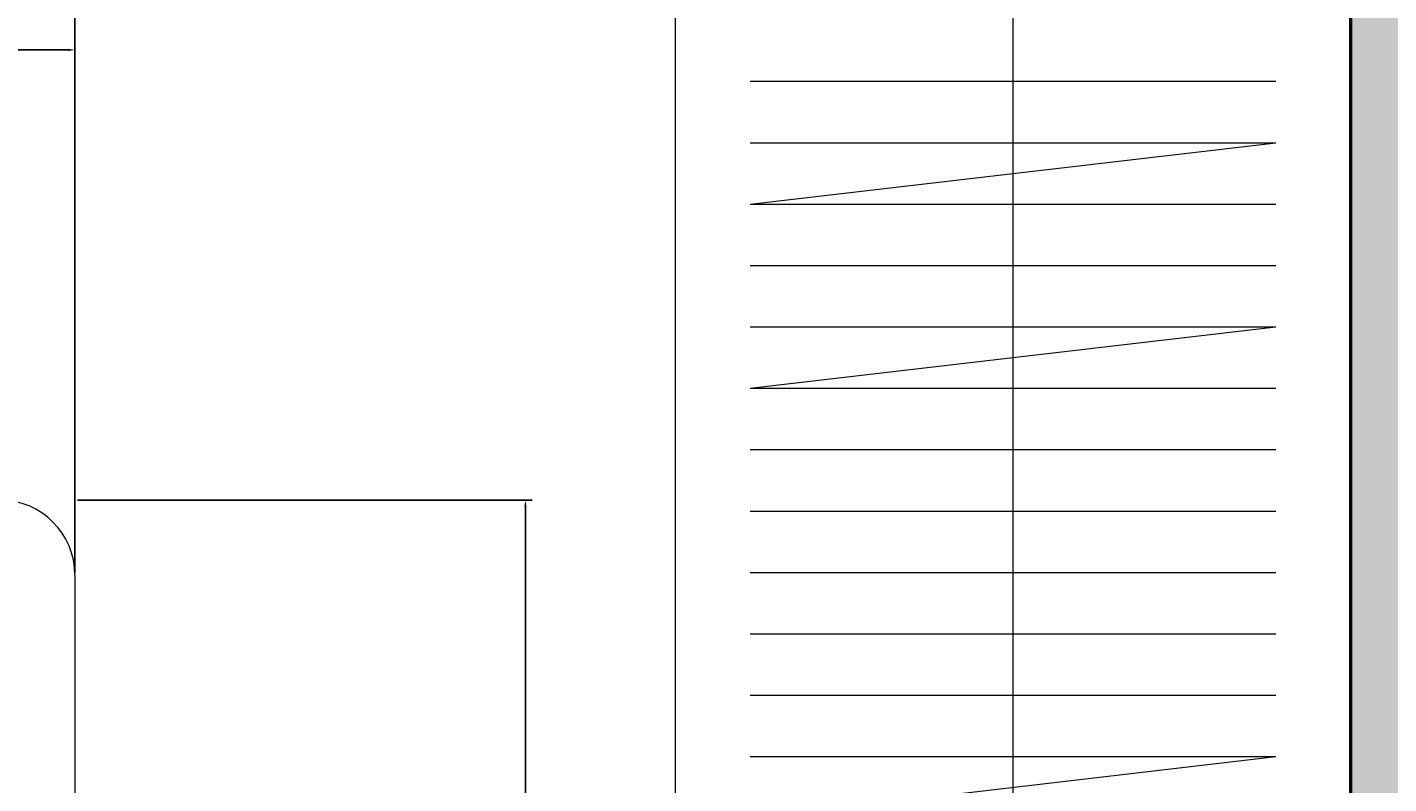
# Model space of a CAD drawing. Units: inches. Extents: x 2307 to 2544, y 2171 to 2540.
# Tile 27 of 52: x 2416 to 2453, y 2485 to 2505. Entities that reach past the tile are written whole.
import ezdxf

# ---------------------------------------------------------------- set-up
doc = ezdxf.new("R2010")
doc.units = ezdxf.units.IN
for name, color, linetype, lineweight in [('A-ANNO-DIMS', 2, 'Continuous', 18), ('A-FLOR-CASE', 9, 'Continuous', 18), ('A-FURN', 8, 'Continuous', 18), ('A-WALL', 7, 'Continuous', 50)]:
    doc.layers.add(name, color=color, linetype=linetype, lineweight=lineweight)
doc.layers.add('A-WALL-PATT', color=18, linetype='Continuous', lineweight=13, true_color=0x000000)
doc.styles.get("Standard").update_dxf_attribs({"font": 'arial.ttf'})
doc.dimstyles.get("Standard").update_dxf_attribs({"dimtxt": 0.18, "dimasz": 0.18, "dimexe": 0.18, "dimexo": 0.0625, "dimgap": 0.09, "dimtad": 0, "dimtih": 1, "dimtoh": 1, "dimdec": 4, "dimzin": 0, "dimdsep": 46, "dimtxsty": 'Standard', "dimcen": 0.09, "dimadec": 0, "dimazin": 0, "dimtfac": 1, "dimtdec": 4, "dimtofl": 0, "dimtmove": 0, "dimatfit": 3, "dimfxl": 1, "dimtolj": 1, "dimtzin": 0, "dimarcsym": 0})

# ---------------------------------------------------------------- blocks, each defined once
blk = doc.blocks.new('Bed - Queen')
blk.add_line((57.99999, -80.00003), (2, -80.00003))
blk.add_arc((57.99999, -78.00003), 2, 270, 0)
blk = doc.blocks.new('WARDROBE-72X18IN')
for p, q in [((0, 72), (0, 0)), ((9, 72), (9, 0)), ((18, 0), (18, 72)), ((16, 63.818), (2, 63.818)), ((16, 62.181), (2, 62.181)), ((16, 62.181), (2, 60.545)), ((16, 60.545), (2, 60.545)), ((16, 58.909), (2, 58.909)), ((16, 57.272), (2, 57.272)), ((16, 57.272), (2, 55.636)), ((16, 55.636), (2, 55.636)), ((16, 54), (2, 54)), ((16, 52.363), (2, 52.363)), ((16, 50.727), (2, 50.727)), ((16, 49.09), (2, 49.09)), ((16, 47.454), (2, 47.454)), ((16, 45.818), (2, 45.818)), ((16, 45.818), (2, 44.181))]:
    blk.add_line(p, q)
blk = doc.blocks.new('*D26')
at = {"layer": 'A-ANNO-DIMS', "color": 0, "lineweight": -2, "transparency": 16777216}
for p, q in [((2337.708, 2492.237), (2337.708, 2504.354)), ((2417.708, 2492.237), (2417.708, 2504.354)), ((2337.888, 2504.174), (2376.714, 2504.174)), ((2417.528, 2504.174), (2378.702, 2504.174))]:
    blk.add_line(p, q, dxfattribs=at)
at = {"layer": 'A-ANNO-DIMS', "color": 0, "transparency": 16777216}
for points in [[(2337.888, 2504.204), (2337.888, 2504.144), (2337.708, 2504.174)], [(2417.528, 2504.204), (2417.528, 2504.144), (2417.708, 2504.174)]]:
    blk.add_solid(points, dxfattribs=at)
at = {"layer": 'Defpoints', "color": 0, "transparency": 16777216}
for p in [(2337.708, 2504.174), (2337.708, 2492.174), (2417.708, 2492.174)]:
    blk.add_point(p, dxfattribs=at)
at = {"layer": 'A-ANNO-DIMS', "color": 0, "transparency": 16777216, "insert": (2377.708, 2504.174), "char_height": 0.18, "attachment_point": 5}
blk.add_mtext('\\A1;QUEEN BED 80', dxfattribs=at)
blk = doc.blocks.new('*D27')
at = {"layer": 'A-ANNO-DIMS', "color": 0, "lineweight": -2, "transparency": 16777216}
for p, q in [((2417.771, 2492.174), (2429.888, 2492.174)), ((2429.708, 2491.994), (2429.708, 2462.356)), ((2429.708, 2432.354), (2429.708, 2461.992)), ((2417.771, 2432.174), (2429.888, 2432.174))]:
    blk.add_line(p, q, dxfattribs=at)
at = {"layer": 'A-ANNO-DIMS', "color": 0, "transparency": 16777216}
for points in [[(2429.678, 2491.994), (2429.738, 2491.994), (2429.708, 2492.174)], [(2429.678, 2432.354), (2429.738, 2432.354), (2429.708, 2432.174)]]:
    blk.add_solid(points, dxfattribs=at)
at = {"layer": 'Defpoints', "color": 0, "transparency": 16777216}
for p in [(2417.708, 2492.174), (2429.708, 2492.174), (2417.708, 2432.174)]:
    blk.add_point(p, dxfattribs=at)
at = {"layer": 'A-ANNO-DIMS', "color": 0, "transparency": 16777216, "insert": (2429.708, 2462.174), "char_height": 0.18, "attachment_point": 5}
blk.add_mtext('\\A1;60', dxfattribs=at)
blk = doc.blocks.new('*D48')
at = {"layer": 'A-ANNO-DIMS', "color": 0, "lineweight": -2, "transparency": 16777216}
for p, q in [((2455.633, 2511.51), (2307.366, 2511.51)), ((2307.546, 2511.33), (2307.546, 2475.69)), ((2307.546, 2439.69), (2307.546, 2475.329)), ((2455.633, 2439.51), (2307.366, 2439.51))]:
    blk.add_line(p, q, dxfattribs=at)
at = {"layer": 'A-ANNO-DIMS', "color": 0, "transparency": 16777216}
for points in [[(2307.516, 2511.33), (2307.576, 2511.33), (2307.546, 2511.51)], [(2307.516, 2439.69), (2307.576, 2439.69), (2307.546, 2439.51)]]:
    blk.add_solid(points, dxfattribs=at)
at = {"layer": 'Defpoints', "color": 0, "transparency": 16777216}
for p in [(2307.546, 2511.51), (2455.696, 2511.51), (2455.696, 2439.51)]:
    blk.add_point(p, dxfattribs=at)
at = {"layer": 'A-ANNO-DIMS', "color": 0, "transparency": 16777216, "insert": (2307.546, 2475.51), "char_height": 0.18, "attachment_point": 5}
blk.add_mtext('\\A1;72', dxfattribs=at)
blk = doc.blocks.new('*D69')
at = {"layer": 'A-ANNO-DIMS', "color": 0, "lineweight": -2, "transparency": 16777216}
for p, q in [((2417.708, 2490.237), (2417.708, 2540.345)), ((2417.888, 2540.165), (2425.247, 2540.165)), ((2433.516, 2540.165), (2426.157, 2540.165)), ((2433.696, 2511.572), (2433.696, 2540.345))]:
    blk.add_line(p, q, dxfattribs=at)
at = {"layer": 'A-ANNO-DIMS', "color": 0, "transparency": 16777216}
for points in [[(2417.888, 2540.195), (2417.888, 2540.135), (2417.708, 2540.165)], [(2433.516, 2540.195), (2433.516, 2540.135), (2433.696, 2540.165)]]:
    blk.add_solid(points, dxfattribs=at)
at = {"layer": 'Defpoints', "color": 0, "transparency": 16777216}
for p in [(2433.696, 2540.165), (2433.696, 2511.51), (2417.708, 2490.174)]:
    blk.add_point(p, dxfattribs=at)
at = {"layer": 'A-ANNO-DIMS', "color": 0, "transparency": 16777216, "insert": (2425.702, 2540.165), "char_height": 0.18, "attachment_point": 5}
blk.add_mtext('\\A1;15.987', dxfattribs=at)

msp = doc.modelspace()

# ---------------------------------------------------------------- hatches: boundary and pattern name
at = {"layer": 'A-WALL-PATT'}
h = msp.add_hatch(color=256, dxfattribs=at)
h.dxf.hatch_style = 1
h.paths.add_polyline_path([(2433.6935, 2199.5096), (2415.6423, 2199.5096), (2415.6423, 2190.5096), (2433.7832, 2190.5096)], flags=17)
h.paths.add_polyline_path([(2367.6423, 2199.5096), (2335.6958, 2199.5096), (2335.6958, 2307.3983), (2326.6958, 2307.3983), (2326.6958, 2190.5096), (2367.6423, 2190.5096)])
h.paths.add_polyline_path([(2524.6958, 2520.5096), (2496.7832, 2520.5096), (2496.7832, 2515.5149), (2472.7832, 2515.5149), (2472.7832, 2520.5096), (2415.4028, 2520.5096), (2415.4028, 2511.5096), (2451.6958, 2511.5096), (2451.6958, 2439.5096), (2451.6958, 2391.5096), (2445.6958, 2391.5096), (2445.6958, 2387.5096), (2455.6958, 2387.5096), (2455.6958, 2435.5096), (2461.6958, 2435.5096), (2461.6958, 2439.5096), (2455.6958, 2439.5096), (2455.6958, 2511.5096), (2515.6958, 2511.5096), (2515.6958, 2439.5096), (2491.6958, 2439.5096), (2491.6958, 2435.5096), (2515.6958, 2435.5096), (2515.6958, 2319.5096), (2451.6958, 2319.5096), (2451.6958, 2281.5096), (2481.6958, 2281.5096), (2481.6958, 2225.5096), (2485.6958, 2225.5096), (2485.6958, 2285.5096), (2455.6958, 2285.5096), (2455.6958, 2315.5096), (2515.6958, 2315.5096), (2515.6958, 2199.5096), (2469.6952, 2199.5096), (2469.785, 2190.5096), (2524.6958, 2190.5096)])

# ---------------------------------------------------------------- linework, layer by layer
at = {"layer": 'A-WALL'}
msp.add_line((2451.6958, 2391.5096), (2451.6958, 2511.5096), dxfattribs=at)

# ---------------------------------------------------------------- block references
at = {"layer": 'A-FLOR-CASE'}
msp.add_blockref('WARDROBE-72X18IN', (2433.696, 2439.51), dxfattribs=at)
at = {"layer": 'A-FURN', "rotation": 90}
msp.add_blockref('Bed - Queen', (2337.7083, 2432.1742), dxfattribs=at)

# ---------------------------------------------------------------- dimensions: what is measured, and where the dimension line sits
at = {"layer": 'A-ANNO-DIMS'}
dim = msp.add_linear_dim(base=(2433.6958, 2540.1649), p1=(2417.7084, 2490.1742), p2=(2433.6958, 2511.5096), dimstyle='Standard', override={"dimdec": 3, "dimlfac": 1, "dimrnd": 0, "dimzin": 0, "dimdsep": 46, "dimlunit": 2}, dxfattribs=at)
dim.commit()
dim.dimension.update_dxf_attribs({"geometry": '*D69', "text_midpoint": (2425.7021, 2540.1649)})
for base, p1, p2, picture, middle in [((2307.5458, 2511.5096), (2455.6958, 2439.5096), (2455.6958, 2511.5096), '*D48', (2307.5458, 2475.5096)), ((2429.7084, 2492.1742), (2417.7084, 2432.1742), (2417.7084, 2492.1742), '*D27', (2429.7084, 2462.1742))]:
    dim = msp.add_linear_dim(base=base, p1=p1, p2=p2, angle=90, dimstyle='Standard', override={"dimdec": 0, "dimlfac": 1, "dimrnd": 0, "dimzin": 0, "dimdsep": 46, "dimlunit": 2}, dxfattribs=at)
    dim.commit()
    dim.dimension.update_dxf_attribs({"geometry": picture, "text_midpoint": middle})
dim = msp.add_linear_dim(base=(2337.7083, 2504.1742), p1=(2417.7084, 2492.1742), p2=(2337.7083, 2492.1742), angle=180, text='QUEEN BED <>', dimstyle='Standard', override={"dimdec": 0, "dimlfac": 1, "dimrnd": 0, "dimzin": 0, "dimdsep": 46, "dimlunit": 2}, dxfattribs=at)
dim.commit()
dim.dimension.update_dxf_attribs({"geometry": '*D26', "text_midpoint": (2377.7083, 2504.1742)})

doc.saveas('drawing.dxf')
